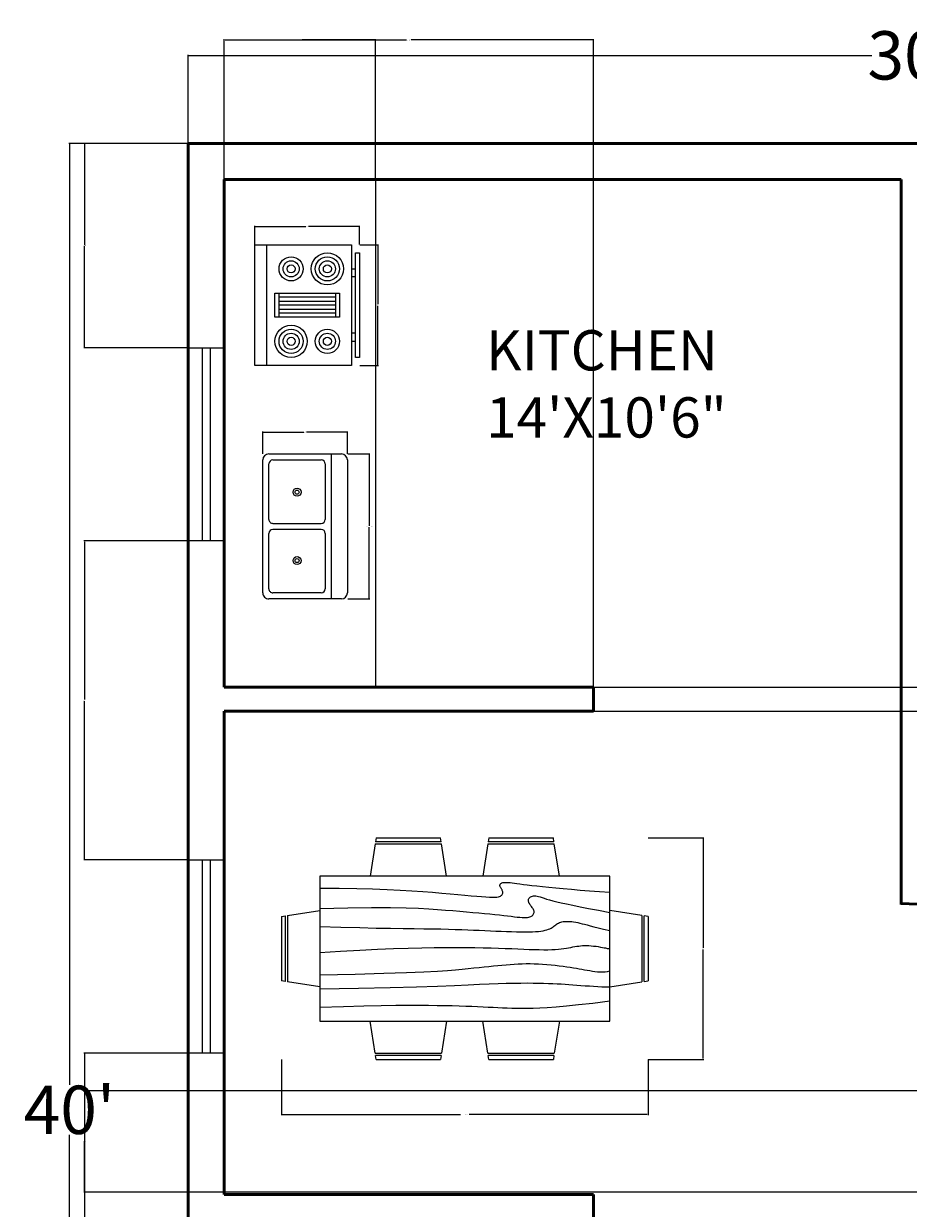
# Model space of a CAD drawing. Units: inches. Extents: x 471 to 898, y -3 to 533.
# Tile 2 of 3: x 471 to 691, y 239 to 533. Entities that reach past the tile are written whole.
import ezdxf

# ---------------------------------------------------------------- set-up
doc = ezdxf.new("R2010")
doc.units = ezdxf.units.IN
doc.header["$MEASUREMENT"] = 0
for name, color, linetype, lineweight in [('A-ANNO-DIMS', 2, 'Continuous', 18), ('A-AREA-IDEN', 7, 'Continuous', 25), ('A-EQPM', 8, 'Continuous', 18), ('A-FLOR-CASE', 8, 'Continuous', 25), ('A-FLOR-FIXT', 9, 'Continuous', 18), ('A-FURN', 8, 'Continuous', 18), ('A-GLAZ', 4, 'Continuous', 18), ('A-WALL', 7, 'Continuous', 50)]:
    doc.layers.add(name, color=color, linetype=linetype, lineweight=lineweight)
doc.styles.get("Standard").update_dxf_attribs({"font": 'arial.ttf'})
doc.dimstyles.get("Standard").update_dxf_attribs({"dimtxt": 0.18, "dimasz": 0.18, "dimexe": 0.18, "dimexo": 0.0625, "dimgap": 0.09, "dimtad": 0, "dimtih": 1, "dimtoh": 1, "dimdec": 1, "dimzin": 0, "dimdsep": 46, "dimlunit": 4, "dimtxsty": 'Standard', "dimcen": 0.09, "dimadec": 0, "dimazin": 0, "dimtfac": 1, "dimtdec": 1, "dimtofl": 0, "dimtmove": 0, "dimatfit": 3, "dimfxl": 1, "dimtolj": 1, "dimtzin": 0, "dimarcsym": 0})

# ---------------------------------------------------------------- blocks, each defined once
blk = doc.blocks.new('Range-Oven - 30 in top')
for p, q in [((0, -3), (30, -3)), ((12, -6), (18, -6)), ((13, -20), (13, -6)), ((14, -6), (14, -20)), ((15, -20), (15, -6)), ((16, -6), (16, -20)), ((17, -20), (17, -6)), ((18, -20), (12, -20)), ((6, -24), (6, -25)), ((8, -25), (8, -24)), ((22, -25), (22, -24)), ((24, -24), (24, -25))]:
    blk.add_line(p, q)
for points in [[(0, -24), (0, 0), (30, 0), (30, -24)], [(12, -21), (12, -5), (18, -5), (18, -21)], [(2, -26), (2, -25), (28, -25), (28, -26)]]:
    blk.add_lwpolyline(points, close=True)
for centre, radius in [((6, -9), 4), ((6, -9), 3), ((6, -9), 2), ((6, -9), 1), ((24, -9), 3), ((24, -9), 2), ((24, -9), 1), ((24, -18), 4), ((6, -18), 3), ((6, -18), 2), ((6, -18), 1), ((24, -18), 3), ((24, -18), 2), ((24, -18), 1)]:
    blk.add_circle(centre, radius)
blk = doc.blocks.new('Sink-double - 36 in top')
for p, q in [((-18, -4), (18, -4)), ((-0.75, -18.5), (-0.75, -6.5)), ((0.75, -6.5), (0.75, -18.5))]:
    blk.add_line(p, q)
for points in [[(-16.5, 0), (16.5, 0)], [(-18, -19.5), (-18, -1.5)], [(18, -1.5), (18, -19.5)], [(-15.5, -5.5), (-1.75, -5.5)], [(1.75, -5.5), (15.5, -5.5)], [(-16.5, -18.5), (-16.5, -6.5)], [(16.5, -6.5), (16.5, -18.5)], [(-1.75, -19.5), (-15.5, -19.5)], [(15.5, -19.5), (1.75, -19.5)], [(16.5, -21), (-16.5, -21)]]:
    blk.add_lwpolyline(points)
for centre, radius in [((-8.5, -12.5), 1), ((8.5, -12.5), 1), ((-8.5, -12.5), 0.5), ((8.5, -12.5), 0.5)]:
    blk.add_circle(centre, radius)
for centre, radius, start, end in [((-16.5, -1.5), 1.5, 90, 180), ((16.5, -1.5), 1.5, 0, 90), ((-15.5, -6.5), 1, 90, 180), ((-1.75, -6.5), 1, 0, 90), ((1.75, -6.5), 1, 90, 180), ((15.5, -6.5), 1, 0, 90), ((-16.5, -19.5), 1.5, 180, 270), ((-15.5, -18.5), 1, 180, 270), ((-1.75, -18.5), 1, 270, 0), ((1.75, -18.5), 1, 180, 270), ((15.5, -18.5), 1, 270, 0), ((16.5, -19.5), 1.5, 270, 0)]:
    blk.add_arc(centre, radius, start, end)
blk = doc.blocks.new('Dining Set - 36 x 72 in.')
for p, q in [((-22, 27.5), (-22.1562, 26.50042)), ((-5.8416, 26.5), (-22.1534, 26.5)), ((-22, 27.5), (-6, 27.5)), ((-5.8437, 26.49966), (-6, 27.5)), ((6, 27.5), (5.8438, 26.50042)), ((22.1584, 26.5), (5.8466, 26.5)), ((6, 27.5), (22, 27.5)), ((22.1563, 26.49966), (22, 27.5)), ((-22.2343, 26.00059), (-23.4847, 17.99762)), ((-22.2304, 26), (-5.7608, 26)), ((-4.5152, 17.99762), (-5.7655, 25.99926)), ((5.7657, 26.00059), (4.5153, 17.99762)), ((5.7696, 26), (22.2392, 26)), ((23.4848, 17.99762), (22.2345, 25.99926)), ((36, 18), (-36, 18)), ((-36, 18), (-36, -18)), ((36, -18), (36, 18)), ((-44.0006, 8.23428), (-35.9976, 9.48474)), ((44.0006, 8.23428), (35.9976, 9.48474)), ((-45.5, 8), (-44.5004, 8.15617)), ((-45.5, 8), (-45.5, -8)), ((-44.5, -8.15843), (-44.5, 8.15338)), ((-44, 8.23041), (-44, -8.23915)), ((44, 8.23041), (44, -8.23915)), ((44.5, -8.15843), (44.5, 8.15338)), ((45.5, 8), (44.5005, 8.15617)), ((45.5, 8), (45.5, -8)), ((-44.4997, -8.15631), (-45.5, -8)), ((-35.9976, -9.48476), (-43.9993, -8.2345)), ((35.9976, -9.48476), (43.9993, -8.2345)), ((44.4997, -8.15631), (45.5, -8)), ((-36, -18), (36, -18)), ((-22.2343, -26.0006), (-23.4847, -17.99762)), ((-4.5152, -17.99762), (-5.7655, -25.99928)), ((5.7657, -26.0006), (4.5153, -17.99762)), ((23.4848, -17.99762), (22.2345, -25.99928)), ((-22.2304, -26), (-5.7608, -26)), ((5.7696, -26), (22.2392, -26)), ((-22, -27.5), (-22.1562, -26.50044)), ((-5.8416, -26.5), (-22.1534, -26.5)), ((-22, -27.5), (-6, -27.5)), ((-5.8437, -26.49967), (-6, -27.5)), ((6, -27.5), (5.8438, -26.50044)), ((22.1584, -26.5), (5.8466, -26.5)), ((6, -27.5), (22, -27.5)), ((22.1563, -26.49967), (22, -27.5))]:
    blk.add_line(p, q)
for points in [[(-36, 15), (-31.1772, 14.97754), (-26.8079, 14.91406), (-22.8538, 14.81543), (-19.276, 14.6875), (-16.0362, 14.53613), (-13.0957, 14.36718), (-10.4159, 14.18652), (-7.9583, 14), (-5.6904, 13.81315), (-3.6035, 13.63021), (-1.6954, 13.45508), (0.0365, 13.29166), (1.5945, 13.14388), (2.9811, 13.01562), (4.1988, 12.9108), (5.25, 12.83333), (6.1393, 12.78613), (6.8802, 12.76823), (7.4883, 12.77767), (7.9792, 12.8125), (8.3685, 12.87077), (8.6719, 12.95052), (8.9049, 13.0498), (9.0833, 13.16666), (9.2205, 13.29899), (9.3216, 13.44401), (9.3895, 13.59879), (9.4271, 13.76041), (9.4373, 13.92594), (9.4232, 14.09245), (9.3875, 14.257), (9.3333, 14.41666), (9.2638, 14.56917), (9.1836, 14.71484), (9.0975, 14.85465), (9.0104, 14.98958), (8.9272, 15.1206), (8.8529, 15.2487), (8.7922, 15.37483), (8.75, 15.5), (8.7305, 15.62467), (8.7344, 15.74739), (8.7617, 15.86621), (8.8125, 15.97916), (8.8867, 16.08431), (8.9844, 16.17968), (9.1055, 16.26334), (9.25, 16.33333), (9.4189, 16.38802), (9.6172, 16.42708), (9.8506, 16.45052), (10.125, 16.45833), (10.4463, 16.45052), (10.8203, 16.42708), (11.2529, 16.38802), (11.75, 16.33333), (12.3184, 16.26318), (12.9694, 16.17838), (13.7151, 16.07991), (14.5677, 15.96875), (15.5395, 15.84586), (16.6426, 15.71224), (17.8893, 15.56884), (19.2917, 15.41666), (20.859, 15.25667), (22.5879, 15.08984), (24.4721, 14.91715), (26.5052, 14.73958), (28.6809, 14.5581), (30.9929, 14.3737), (33.4347, 14.18733), (36, 14)], [(-36, 10), (-28.9766, 10.14274), (-23.1725, 10.20442), (-18.4241, 10.19775), (-14.5677, 10.13541), (-11.4399, 10.03011), (-8.877, 9.89453), (-6.7154, 9.74137), (-4.7917, 9.58333), (-2.9698, 9.43082), (-1.2246, 9.28515), (0.4415, 9.14534), (2.026, 9.01041), (3.5266, 8.87939), (4.9408, 8.7513), (6.266, 8.62516), (7.5, 8.5), (8.6411, 8.37549), (9.6914, 8.2539), (10.6538, 8.13818), (11.5312, 8.03125), (12.3267, 7.93603), (13.043, 7.85547), (13.6831, 7.79248), (14.25, 7.75), (14.7471, 7.7303), (15.1797, 7.73307), (15.5537, 7.75732), (15.875, 7.80208), (16.1494, 7.86637), (16.3828, 7.94922), (16.5811, 8.04964), (16.75, 8.16666), (16.8944, 8.29915), (17.0143, 8.44531), (17.1089, 8.60319), (17.1771, 8.77083), (17.218, 8.94629), (17.2305, 9.1276), (17.2137, 9.31282), (17.1667, 9.5), (17.0895, 9.6875), (16.987, 9.875), (16.8649, 10.0625), (16.7292, 10.25), (16.5856, 10.4375), (16.4401, 10.625), (16.2985, 10.8125), (16.1667, 11), (16.05, 11.18733), (15.9518, 11.3737), (15.8752, 11.5581), (15.8229, 11.73958), (15.798, 11.91715), (15.8034, 12.08984), (15.842, 12.25667), (15.9167, 12.41666), (16.0295, 12.56836), (16.1784, 12.70833), (16.3605, 12.83268), (16.5729, 12.9375), (16.8127, 13.01888), (17.0768, 13.07291), (17.3625, 13.0957), (17.6667, 13.08333), (17.9894, 13.03312), (18.3418, 12.94726), (18.7382, 12.82918), (19.1927, 12.68229), (19.7195, 12.51001), (20.3327, 12.31575), (21.0465, 12.10294), (21.875, 11.875), (22.8357, 11.63354), (23.959, 11.37304), (25.2786, 11.08618), (26.8282, 10.76562), (28.6414, 10.40405), (30.752, 9.99414), (33.1936, 9.52856), (36, 9)], [(-36, 5.5), (-30.7157, 5.3348), (-26.069, 5.20963), (-21.9946, 5.11767), (-18.4271, 5.05208), (-15.3009, 5.00602), (-12.5508, 4.97265), (-10.1112, 4.94515), (-7.9167, 4.91666), (-5.909, 4.88167), (-4.0586, 4.83984), (-2.3429, 4.79215), (-0.7396, 4.73958), (0.7739, 4.6831), (2.22, 4.6237), (3.6213, 4.56233), (5, 4.5), (6.373, 4.43782), (7.7344, 4.3776), (9.0723, 4.32129), (10.375, 4.27083), (11.6309, 4.22819), (12.8281, 4.19531), (13.9551, 4.17415), (15, 4.16666), (15.954, 4.17448), (16.819, 4.19791), (17.6001, 4.23698), (18.3021, 4.29166), (18.9299, 4.36198), (19.4883, 4.44791), (19.9823, 4.54948), (20.4167, 4.66666), (20.7969, 4.79899), (21.1302, 4.94401), (21.4245, 5.09879), (21.6875, 5.26041), (21.9271, 5.42594), (22.1511, 5.59245), (22.3672, 5.757), (22.5834, 5.91666), (22.8065, 6.06868), (23.0404, 6.21093), (23.2879, 6.34147), (23.5521, 6.45833), (23.8358, 6.55957), (24.142, 6.64323), (24.4735, 6.70735), (24.8334, 6.75), (25.2235, 6.76969), (25.642, 6.76692), (26.0858, 6.74267), (26.5521, 6.69791), (27.0379, 6.63362), (27.5404, 6.55078), (28.0565, 6.45036), (28.5834, 6.33333), (29.1242, 6.19987), (29.7071, 6.04687), (30.3661, 5.87044), (31.1354, 5.66666), (32.0493, 5.43164), (33.142, 5.16146), (34.4475, 4.85221), (36, 4.5)], [(-36, -1), (-30.7915, -0.6591), (-26.0195, -0.38216), (-21.6519, -0.16284), (-17.6563, 0.00521), (-14.0005, 0.12833), (-10.6523, 0.21289), (-7.5796, 0.26522), (-4.75, 0.29166), (-2.134, 0.29793), (0.2878, 0.28711), (2.5317, 0.26163), (4.6146, 0.22396), (6.5529, 0.17651), (8.3633, 0.12174), (10.0623, 0.06209), (11.6667, 0), (13.1899, -0.06201), (14.6341, -0.1211), (15.9982, -0.17432), (17.2813, -0.21875), (18.4823, -0.25147), (19.6003, -0.26953), (20.6343, -0.27002), (21.5834, -0.25), (22.4481, -0.20768), (23.2357, -0.14584), (23.9549, -0.06836), (24.6146, 0.02083), (25.2235, 0.11784), (25.7904, 0.21875), (26.3241, 0.31966), (26.8334, 0.41666), (27.3265, 0.50618), (27.8099, 0.58593), (28.2894, 0.65397), (28.7709, 0.70833), (29.2601, 0.74707), (29.763, 0.76823), (30.2855, 0.76985), (30.8334, 0.75), (31.4088, 0.70784), (31.9994, 0.64713), (32.589, 0.57275), (33.1615, 0.48958), (33.7008, 0.4025), (34.1908, 0.3164), (34.6153, 0.23616), (34.9584, 0.16666), (35.2099, 0.11165), (35.3848, 0.07031), (35.504, 0.04069), (35.5886, 0.02083), (35.6594, 0.00879), (35.7377, 0.0026), (35.8442, 0.00032), (36, 0)], [(-36, -6.5), (-27.1843, -6.31267), (-20.084, -6.1263), (-14.469, -5.9419), (-10.1094, -5.76042), (-6.7752, -5.58285), (-4.2363, -5.41016), (-2.2629, -5.24333), (-0.625, -5.08334), (0.8708, -4.93099), (2.2715, -4.78646), (3.5872, -4.64974), (4.8281, -4.52084), (6.0046, -4.39974), (7.127, -4.28646), (8.2053, -4.18099), (9.25, -4.08334), (10.2705, -3.99382), (11.2734, -3.91407), (12.2647, -3.84603), (13.25, -3.79167), (14.2354, -3.75293), (15.2266, -3.73177), (16.2295, -3.73015), (17.25, -3.75), (18.2912, -3.79248), (19.3451, -3.85547), (20.4009, -3.93604), (21.4479, -4.03125), (22.4754, -4.13819), (23.4727, -4.25391), (24.4289, -4.37549), (25.3334, -4.5), (26.1785, -4.62492), (26.9694, -4.74935), (27.7145, -4.87281), (28.4219, -4.99479), (29.1, -5.11483), (29.7572, -5.23242), (30.4016, -5.34709), (31.0417, -5.45834), (31.6837, -5.56437), (32.3262, -5.65821), (32.9658, -5.73153), (33.599, -5.77604), (34.2224, -5.78345), (34.8327, -5.74545), (35.4264, -5.65373), (36, -5.5)], [(-36, -10), (-26.4022, -9.81299), (-18.4675, -9.62891), (-11.9839, -9.45069), (-6.7396, -9.28125), (-2.5226, -9.12354), (0.8789, -8.98047), (3.6769, -8.85498), (6.0833, -8.75), (8.2767, -8.66765), (10.3021, -8.60677), (12.1712, -8.56543), (13.8958, -8.54167), (15.4876, -8.53353), (16.9583, -8.53907), (18.3197, -8.55632), (19.5834, -8.58334), (20.7616, -8.61841), (21.8685, -8.66081), (22.9188, -8.71004), (23.9271, -8.76563), (24.9081, -8.82707), (25.8763, -8.89388), (26.8465, -8.96558), (27.8334, -9.04167), (28.8474, -9.12118), (29.8828, -9.20117), (30.93, -9.27824), (31.9792, -9.34896), (33.0205, -9.40991), (34.0443, -9.45768), (35.0407, -9.48885), (36, -9.5)], [(-36, -14.5), (-30.0881, -14.33513), (-25.0332, -14.21224), (-20.7312, -14.12647), (-17.0781, -14.07292), (-13.97, -14.04671), (-11.3027, -14.04297), (-8.9724, -14.05681), (-6.875, -14.08334), (-4.9224, -14.11833), (-3.0905, -14.16016), (-1.3709, -14.20785), (0.2448, -14.26042), (1.7647, -14.3169), (3.1973, -14.3763), (4.5507, -14.43767), (5.8333, -14.5), (7.0554, -14.5621), (8.235, -14.62175), (9.3922, -14.67652), (10.5469, -14.72396), (11.7192, -14.76164), (12.929, -14.78711), (14.1965, -14.79794), (15.5417, -14.79167), (16.9933, -14.76424), (18.6152, -14.70508), (20.4804, -14.60197), (22.6615, -14.44271), (25.2312, -14.21509), (28.2624, -13.9069), (31.8277, -13.50594), (36, -13)]]:
    blk.add_lwpolyline(points)
blk = doc.blocks.new('*D12')
at = {"layer": 'A-ANNO-DIMS', "color": 0, "lineweight": -2, "transparency": 16777216}
for p, q in [((512.23, 503.14), (512.23, 525.11)), ((512.41, 524.93), (681.96, 524.93)), ((872.05, 524.93), (702.5, 524.93)), ((872.23, 503.14), (872.23, 525.11))]:
    blk.add_line(p, q, dxfattribs=at)
at = {"layer": 'A-ANNO-DIMS', "color": 0, "transparency": 16777216}
for points in [[(512.41, 524.96), (512.41, 524.9), (512.23, 524.93)], [(872.05, 524.96), (872.05, 524.9), (872.23, 524.93)]]:
    blk.add_solid(points, dxfattribs=at)
at = {"layer": 'Defpoints', "color": 0, "transparency": 16777216}
for p in [(872.23, 524.93), (512.23, 503.07), (872.23, 503.07)]:
    blk.add_point(p, dxfattribs=at)
at = {"layer": 'A-ANNO-DIMS', "color": 0, "transparency": 16777216, "insert": (692.23, 524.93), "char_height": 12, "attachment_point": 5}
blk.add_mtext("\\A1;30'", dxfattribs=at)
blk = doc.blocks.new('*D13')
at = {"layer": 'A-ANNO-DIMS', "color": 0, "lineweight": -2, "transparency": 16777216}
for p, q in [((512.17, 503.07), (482.62, 503.07)), ((482.8, 502.89), (482.8, 269.29)), ((482.8, 23.25), (482.8, 256.86)), ((512.17, 23.07), (482.62, 23.07))]:
    blk.add_line(p, q, dxfattribs=at)
at = {"layer": 'A-ANNO-DIMS', "color": 0, "transparency": 16777216}
for points in [[(482.77, 502.89), (482.83, 502.89), (482.8, 503.07)], [(482.77, 23.25), (482.83, 23.25), (482.8, 23.07)]]:
    blk.add_solid(points, dxfattribs=at)
at = {"layer": 'Defpoints', "color": 0, "transparency": 16777216}
for p in [(512.23, 503.07), (482.8, 23.07), (512.23, 23.07)]:
    blk.add_point(p, dxfattribs=at)
at = {"layer": 'A-ANNO-DIMS', "color": 0, "transparency": 16777216, "insert": (482.8, 263.07), "char_height": 12, "attachment_point": 5}
blk.add_mtext("\\A1;40'", dxfattribs=at)
blk = doc.blocks.new('WIN-48X9')
for p, q in [((0, 48), (9, 48)), ((0, 0), (0, 48)), ((3.5, 48), (3.5, 0)), ((5.5, 48), (5.5, 0)), ((9, 48), (9, 0)), ((9, 0), (0, 0))]:
    blk.add_line(p, q)
blk = doc.blocks.new('*D23')
at = {"layer": 'A-ANNO-DIMS', "color": 0, "lineweight": -2, "transparency": 16777216}
for p, q in [((554.87, 477.92), (559.49, 477.92)), ((559.31, 477.74), (559.31, 463.11)), ((559.31, 448.1), (559.31, 462.74)), ((554.87, 447.92), (559.49, 447.92))]:
    blk.add_line(p, q, dxfattribs=at)
at = {"layer": 'A-ANNO-DIMS', "color": 0, "transparency": 16777216}
for points in [[(559.28, 477.74), (559.34, 477.74), (559.31, 477.92)], [(559.28, 448.1), (559.34, 448.1), (559.31, 447.92)]]:
    blk.add_solid(points, dxfattribs=at)
at = {"layer": 'Defpoints', "color": 0, "transparency": 16777216}
for p in [(554.81, 477.92), (559.31, 477.92), (554.81, 447.92)]:
    blk.add_point(p, dxfattribs=at)
at = {"layer": 'A-ANNO-DIMS', "color": 0, "transparency": 16777216, "insert": (559.31, 462.92), "char_height": 0.18, "attachment_point": 5}
blk.add_mtext('\\A1;RANGE 2\'-6"', dxfattribs=at)
blk = doc.blocks.new('*D24')
at = {"layer": 'A-ANNO-DIMS', "color": 0, "lineweight": -2, "transparency": 16777216}
for p, q in [((528.81, 477.99), (528.81, 482.6)), ((554.81, 477.99), (554.81, 482.6)), ((528.99, 482.42), (541.48, 482.42)), ((554.63, 482.42), (542.14, 482.42))]:
    blk.add_line(p, q, dxfattribs=at)
at = {"layer": 'A-ANNO-DIMS', "color": 0, "transparency": 16777216}
for points in [[(528.99, 482.45), (528.99, 482.39), (528.81, 482.42)], [(554.63, 482.45), (554.63, 482.39), (554.81, 482.42)]]:
    blk.add_solid(points, dxfattribs=at)
at = {"layer": 'Defpoints', "color": 0, "transparency": 16777216}
for p in [(528.81, 482.42), (528.81, 477.92), (554.81, 477.92)]:
    blk.add_point(p, dxfattribs=at)
at = {"layer": 'A-ANNO-DIMS', "color": 0, "transparency": 16777216, "insert": (541.81, 482.42), "char_height": 0.18, "attachment_point": 5}
blk.add_mtext('\\A1;2\'-2"', dxfattribs=at)
blk = doc.blocks.new('*D25')
at = {"layer": 'A-ANNO-DIMS', "color": 0, "lineweight": -2, "transparency": 16777216}
for p, q in [((551.85, 425.96), (557.37, 425.96)), ((557.19, 425.78), (557.19, 408.14)), ((557.19, 390.14), (557.19, 407.78)), ((551.85, 389.96), (557.37, 389.96))]:
    blk.add_line(p, q, dxfattribs=at)
at = {"layer": 'A-ANNO-DIMS', "color": 0, "transparency": 16777216}
for points in [[(557.16, 425.78), (557.22, 425.78), (557.19, 425.96)], [(557.16, 390.14), (557.22, 390.14), (557.19, 389.96)]]:
    blk.add_solid(points, dxfattribs=at)
at = {"layer": 'Defpoints', "color": 0, "transparency": 16777216}
for p in [(551.79, 425.96), (551.79, 389.96), (557.19, 389.96)]:
    blk.add_point(p, dxfattribs=at)
at = {"layer": 'A-ANNO-DIMS', "color": 0, "transparency": 16777216, "insert": (557.19, 407.96), "char_height": 0.18, "attachment_point": 5}
blk.add_mtext('\\A1;DOUBLE SINK 3\'-0"', dxfattribs=at)
blk = doc.blocks.new('*D26')
at = {"layer": 'A-ANNO-DIMS', "color": 0, "lineweight": -2, "transparency": 16777216}
for p, q in [((530.79, 426.02), (530.79, 431.54)), ((530.97, 431.36), (540.97, 431.36)), ((551.61, 431.36), (541.61, 431.36)), ((551.79, 426.02), (551.79, 431.54))]:
    blk.add_line(p, q, dxfattribs=at)
at = {"layer": 'A-ANNO-DIMS', "color": 0, "transparency": 16777216}
for points in [[(530.97, 431.39), (530.97, 431.33), (530.79, 431.36)], [(551.61, 431.39), (551.61, 431.33), (551.79, 431.36)]]:
    blk.add_solid(points, dxfattribs=at)
at = {"layer": 'Defpoints', "color": 0, "transparency": 16777216}
for p in [(551.79, 431.36), (530.79, 425.96), (551.79, 425.96)]:
    blk.add_point(p, dxfattribs=at)
at = {"layer": 'A-ANNO-DIMS', "color": 0, "transparency": 16777216, "insert": (541.29, 431.36), "char_height": 0.18, "attachment_point": 5}
blk.add_mtext('\\A1;1\'-9"', dxfattribs=at)
blk = doc.blocks.new('*D29')
at = {"layer": 'A-ANNO-DIMS', "color": 0, "lineweight": -2, "transparency": 16777216}
for p, q in [((535.4, 275.53), (535.4, 261.77)), ((626.4, 275.53), (626.4, 261.77)), ((535.58, 261.95), (579.82, 261.95)), ((626.22, 261.95), (581.98, 261.95))]:
    blk.add_line(p, q, dxfattribs=at)
at = {"layer": 'A-ANNO-DIMS', "color": 0, "transparency": 16777216}
for points in [[(535.58, 261.98), (535.58, 261.92), (535.4, 261.95)], [(626.22, 261.98), (626.22, 261.92), (626.4, 261.95)]]:
    blk.add_solid(points, dxfattribs=at)
at = {"layer": 'Defpoints', "color": 0, "transparency": 16777216}
for p in [(535.4, 275.6), (626.4, 275.6), (626.4, 261.95)]:
    blk.add_point(p, dxfattribs=at)
at = {"layer": 'A-ANNO-DIMS', "color": 0, "transparency": 16777216, "insert": (580.9, 261.95), "char_height": 0.18, "attachment_point": 5}
blk.add_mtext('\\A1;DINING SET 7\'-7"', dxfattribs=at)
blk = doc.blocks.new('*D30')
at = {"layer": 'A-ANNO-DIMS', "color": 0, "lineweight": -2, "transparency": 16777216}
for p, q in [((626.46, 330.6), (640.23, 330.6)), ((640.05, 330.42), (640.05, 303.28)), ((640.05, 275.78), (640.05, 302.92)), ((626.46, 275.6), (640.23, 275.6))]:
    blk.add_line(p, q, dxfattribs=at)
at = {"layer": 'A-ANNO-DIMS', "color": 0, "transparency": 16777216}
for points in [[(640.02, 330.42), (640.08, 330.42), (640.05, 330.6)], [(640.02, 275.78), (640.08, 275.78), (640.05, 275.6)]]:
    blk.add_solid(points, dxfattribs=at)
at = {"layer": 'Defpoints', "color": 0, "transparency": 16777216}
for p in [(626.4, 330.6), (640.05, 330.6), (626.4, 275.6)]:
    blk.add_point(p, dxfattribs=at)
at = {"layer": 'A-ANNO-DIMS', "color": 0, "transparency": 16777216, "insert": (640.05, 303.1), "char_height": 0.18, "attachment_point": 5}
blk.add_mtext('\\A1;4\'-7"', dxfattribs=at)
blk = doc.blocks.new('*D35')
at = {"layer": 'A-ANNO-DIMS', "color": 0, "lineweight": -2, "transparency": 16777216}
for p, q in [((512.17, 503.07), (486.35, 503.07)), ((486.53, 502.89), (486.53, 477.89)), ((486.53, 452.52), (486.53, 477.52)), ((512.17, 452.34), (486.35, 452.34))]:
    blk.add_line(p, q, dxfattribs=at)
at = {"layer": 'A-ANNO-DIMS', "color": 0, "transparency": 16777216}
for points in [[(486.5, 502.89), (486.56, 502.89), (486.53, 503.07)], [(486.5, 452.52), (486.56, 452.52), (486.53, 452.34)]]:
    blk.add_solid(points, dxfattribs=at)
at = {"layer": 'Defpoints', "color": 0, "transparency": 16777216}
for p in [(512.23, 503.07), (486.53, 452.34), (512.23, 452.34)]:
    blk.add_point(p, dxfattribs=at)
at = {"layer": 'A-ANNO-DIMS', "color": 0, "transparency": 16777216, "insert": (486.53, 477.71), "char_height": 0.18, "attachment_point": 5}
blk.add_mtext('\\A1;4\'-2 1/2"', dxfattribs=at)
blk = doc.blocks.new('*D36')
at = {"layer": 'A-ANNO-DIMS', "color": 0, "lineweight": -2, "transparency": 16777216}
for p, q in [((512.17, 404.34), (486.35, 404.34)), ((486.53, 404.16), (486.53, 364.94)), ((486.53, 325.36), (486.53, 364.58)), ((512.17, 325.18), (486.35, 325.18))]:
    blk.add_line(p, q, dxfattribs=at)
at = {"layer": 'A-ANNO-DIMS', "color": 0, "transparency": 16777216}
for points in [[(486.5, 404.16), (486.56, 404.16), (486.53, 404.34)], [(486.5, 325.36), (486.56, 325.36), (486.53, 325.18)]]:
    blk.add_solid(points, dxfattribs=at)
at = {"layer": 'Defpoints', "color": 0, "transparency": 16777216}
for p in [(512.23, 404.34), (486.53, 325.18), (512.23, 325.18)]:
    blk.add_point(p, dxfattribs=at)
at = {"layer": 'A-ANNO-DIMS', "color": 0, "transparency": 16777216, "insert": (486.53, 364.76), "char_height": 0.18, "attachment_point": 5}
blk.add_mtext('\\A1;6\'-7"', dxfattribs=at)
blk = doc.blocks.new('*D37')
at = {"layer": 'A-ANNO-DIMS', "color": 0, "lineweight": -2, "transparency": 16777216}
for p, q in [((512.17, 277.18), (486.35, 277.18)), ((486.53, 277), (486.53, 214.23)), ((486.53, 151.09), (486.53, 213.86)), ((512.17, 150.91), (486.35, 150.91))]:
    blk.add_line(p, q, dxfattribs=at)
at = {"layer": 'A-ANNO-DIMS', "color": 0, "transparency": 16777216}
for points in [[(486.5, 277), (486.56, 277), (486.53, 277.18)], [(486.5, 151.09), (486.56, 151.09), (486.53, 150.91)]]:
    blk.add_solid(points, dxfattribs=at)
at = {"layer": 'Defpoints', "color": 0, "transparency": 16777216}
for p in [(512.23, 277.18), (486.53, 150.91), (512.23, 150.91)]:
    blk.add_point(p, dxfattribs=at)
at = {"layer": 'A-ANNO-DIMS', "color": 0, "transparency": 16777216, "insert": (486.53, 214.04), "char_height": 0.18, "attachment_point": 5}
blk.add_mtext('\\A1;10\'-6 1/2"', dxfattribs=at)
blk = doc.blocks.new('*D44')
at = {"layer": 'A-ANNO-DIMS', "color": 0, "lineweight": -2, "transparency": 16777216}
for p, q in [((521.23, 368.14), (521.23, 528.95)), ((521.41, 528.77), (566.49, 528.77)), ((612.65, 528.77), (567.57, 528.77)), ((612.83, 368.14), (612.83, 528.95))]:
    blk.add_line(p, q, dxfattribs=at)
at = {"layer": 'A-ANNO-DIMS', "color": 0, "transparency": 16777216}
for points in [[(521.41, 528.8), (521.41, 528.74), (521.23, 528.77)], [(612.65, 528.8), (612.65, 528.74), (612.83, 528.77)]]:
    blk.add_solid(points, dxfattribs=at)
at = {"layer": 'Defpoints', "color": 0, "transparency": 16777216}
for p in [(612.83, 528.77), (521.23, 368.07), (612.83, 368.07)]:
    blk.add_point(p, dxfattribs=at)
at = {"layer": 'A-ANNO-DIMS', "color": 0, "transparency": 16777216, "insert": (567.03, 528.77), "char_height": 0.18, "attachment_point": 5}
blk.add_mtext('\\A1;7\'-7 1/2"', dxfattribs=at)
blk = doc.blocks.new('*D45')
at = {"layer": 'A-ANNO-DIMS', "color": 0, "lineweight": -2, "transparency": 16777216}
for p, q in [((612.9, 368.07), (898.15, 368.07)), ((897.97, 367.89), (897.97, 365.26)), ((897.97, 362.25), (897.97, 364.89)), ((612.9, 362.07), (898.15, 362.07))]:
    blk.add_line(p, q, dxfattribs=at)
at = {"layer": 'A-ANNO-DIMS', "color": 0, "transparency": 16777216}
for points in [[(897.94, 367.89), (898, 367.89), (897.97, 368.07)], [(897.94, 362.25), (898, 362.25), (897.97, 362.07)]]:
    blk.add_solid(points, dxfattribs=at)
at = {"layer": 'Defpoints', "color": 0, "transparency": 16777216}
for p in [(612.83, 368.07), (897.97, 368.07), (612.83, 362.07)]:
    blk.add_point(p, dxfattribs=at)
at = {"layer": 'A-ANNO-DIMS', "color": 0, "transparency": 16777216, "insert": (897.97, 365.07), "char_height": 0.18, "attachment_point": 5}
blk.add_mtext('\\A1;0\'-6"', dxfattribs=at)
blk = doc.blocks.new('*D47')
at = {"layer": 'A-ANNO-DIMS', "color": 0, "lineweight": -2, "transparency": 16777216}
for p, q in [((521.23, 494.14), (521.23, 528.95)), ((521.41, 528.77), (539.45, 528.77)), ((558.56, 528.77), (540.53, 528.77)), ((558.74, 494.14), (558.74, 528.95))]:
    blk.add_line(p, q, dxfattribs=at)
at = {"layer": 'A-ANNO-DIMS', "color": 0, "transparency": 16777216}
for points in [[(521.41, 528.8), (521.41, 528.74), (521.23, 528.77)], [(558.56, 528.8), (558.56, 528.74), (558.74, 528.77)]]:
    blk.add_solid(points, dxfattribs=at)
at = {"layer": 'Defpoints', "color": 0, "transparency": 16777216}
for p in [(558.74, 528.77), (521.23, 494.07), (558.74, 494.07)]:
    blk.add_point(p, dxfattribs=at)
at = {"layer": 'A-ANNO-DIMS', "color": 0, "transparency": 16777216, "insert": (539.99, 528.77), "char_height": 0.18, "attachment_point": 5}
blk.add_mtext('\\A1;3\'-1 1/2"', dxfattribs=at)
blk = doc.blocks.new('*D50')
at = {"layer": 'A-ANNO-DIMS', "color": 0, "lineweight": -2, "transparency": 16777216}
for p, q in [((785.17, 267.78), (486.35, 267.78)), ((486.53, 267.6), (486.53, 255.39)), ((486.53, 242.81), (486.53, 255.03)), ((791.03, 242.63), (486.35, 242.63))]:
    blk.add_line(p, q, dxfattribs=at)
at = {"layer": 'A-ANNO-DIMS', "color": 0, "transparency": 16777216}
for points in [[(486.5, 267.6), (486.56, 267.6), (486.53, 267.78)], [(486.5, 242.81), (486.56, 242.81), (486.53, 242.63)]]:
    blk.add_solid(points, dxfattribs=at)
at = {"layer": 'Defpoints', "color": 0, "transparency": 16777216}
for p in [(486.53, 267.78), (785.23, 267.78), (791.1, 242.63)]:
    blk.add_point(p, dxfattribs=at)
at = {"layer": 'A-ANNO-DIMS', "color": 0, "transparency": 16777216, "insert": (486.53, 255.21), "char_height": 0.18, "attachment_point": 5}
blk.add_mtext('\\A1;2\'-1"', dxfattribs=at)

msp = doc.modelspace()

# ---------------------------------------------------------------- linework, layer by layer
at = {"layer": 'A-FLOR-CASE'}
msp.add_line((558.74, 494.07), (558.74, 368.07), dxfattribs=at)
at = {"layer": 'A-WALL'}
for p, q in [((512.23, 23.07), (512.23, 503.07)), ((512.23, 503.07), (872.23, 503.07)), ((521.23, 494.07), (689.23, 494.07)), ((521.23, 494.07), (689.23, 494.07)), ((521.23, 368.07), (521.23, 494.07)), ((689.23, 494.07), (689.23, 320.07)), ((612.83, 368.07), (521.23, 368.07)), ((612.83, 368.07), (612.83, 362.07)), ((612.83, 362.07), (521.23, 362.07)), ((521.23, 242.07), (521.23, 362.07)), ((689.23, 362.07), (689.23, 314.07)), ((695.23, 314.07), (689.23, 314.28)), ((612.83, 242.07), (521.23, 242.07)), ((612.83, 242.07), (612.83, 236.07))]:
    msp.add_line(p, q, dxfattribs=at)

# ---------------------------------------------------------------- block references
at = {"layer": 'A-EQPM', "rotation": 90}
msp.add_blockref('Range-Oven - 30 in top', (528.81, 447.92), dxfattribs=at)
at = {"layer": 'A-FLOR-FIXT', "rotation": 270}
msp.add_blockref('Sink-double - 36 in top', (551.79, 407.96), dxfattribs=at)
at = {"layer": 'A-FURN'}
msp.add_blockref('Dining Set - 36 x 72 in.', (580.9, 303.1), dxfattribs=at)
at = {"layer": 'A-GLAZ'}
for p in [(512.23, 404.34), (512.23, 277.18)]:
    msp.add_blockref('WIN-48X9', p, dxfattribs=at)

# ---------------------------------------------------------------- texts
at = {"layer": 'A-AREA-IDEN', "insert": (586.21, 456.69), "char_height": 10, "attachment_point": 1}
msp.add_mtext_dynamic_manual_height_columns('KITCHEN\\P14\'X10\'6"', width=80.8054, gutter_width=1, heights=[0], dxfattribs=at)

# ---------------------------------------------------------------- dimensions: what is measured, and where the dimension line sits
at = {"layer": 'A-ANNO-DIMS'}
for base, p1, p2, override, picture, middle in [((872.23, 524.93), (512.23, 503.07), (872.23, 503.07), {"dimtxt": 12, "dimclrd": 0, "dimclre": 0, "dimclrt": 0}, '*D12', (692.23, 524.93)), ((612.83, 528.77), (521.23, 368.07), (612.83, 368.07), {"dimdec": 1, "dimlfac": 1, "dimrnd": 0, "dimzin": 1, "dimdsep": 46, "dimlunit": 4, "dimfrac": 2}, '*D44', (567.03, 528.77)), ((558.74, 528.77), (521.23, 494.07), (558.74, 494.07), {"dimdec": 1, "dimlfac": 1, "dimrnd": 0, "dimzin": 1, "dimdsep": 46, "dimlunit": 4, "dimfrac": 2}, '*D47', (539.99, 528.77)), ((551.79, 431.36), (530.79, 425.96), (551.79, 425.96), {"dimdec": 1, "dimlfac": 1, "dimrnd": 0, "dimzin": 1, "dimdsep": 46, "dimlunit": 4, "dimfrac": 2}, '*D26', (541.29, 431.36))]:
    dim = msp.add_linear_dim(base=base, p1=p1, p2=p2, dimstyle='Standard', override=override, dxfattribs=at)
    dim.commit()
    dim.dimension.update_dxf_attribs({"geometry": picture, "text_midpoint": middle})
for base, p1, p2, angle, override, picture, middle in [((482.8, 23.07), (512.23, 503.07), (512.23, 23.07), 90, {"dimtxt": 12, "dimclrd": 0, "dimclre": 0, "dimclrt": 0}, '*D13', (482.8, 263.07)), ((486.53, 452.34), (512.23, 503.07), (512.23, 452.34), 90, {"dimdec": 1, "dimlfac": 1, "dimrnd": 0, "dimzin": 1, "dimdsep": 46, "dimlunit": 4, "dimfrac": 2}, '*D35', (486.53, 477.71)), ((528.81, 482.42), (554.81, 477.92), (528.81, 477.92), 180, {"dimdec": 1, "dimlfac": 1, "dimrnd": 0, "dimzin": 1, "dimdsep": 46, "dimlunit": 4, "dimfrac": 2}, '*D24', (541.81, 482.42)), ((486.53, 325.18), (512.23, 404.34), (512.23, 325.18), 90, {"dimdec": 1, "dimlfac": 1, "dimrnd": 0, "dimzin": 1, "dimdsep": 46, "dimlunit": 4, "dimfrac": 2}, '*D36', (486.53, 364.76)), ((897.97, 368.07), (612.83, 362.07), (612.83, 368.07), 90, {"dimdec": 1, "dimlfac": 1, "dimrnd": 0, "dimzin": 1, "dimdsep": 46, "dimlunit": 4, "dimfrac": 2}, '*D45', (897.97, 365.07)), ((640.05, 330.6), (626.4, 275.6), (626.4, 330.6), 90, {"dimdec": 1, "dimlfac": 1, "dimrnd": 0, "dimzin": 1, "dimdsep": 46, "dimlunit": 4, "dimfrac": 2}, '*D30', (640.05, 303.1)), ((486.53, 150.91), (512.23, 277.18), (512.23, 150.91), 90, {"dimdec": 1, "dimlfac": 1, "dimrnd": 0, "dimzin": 1, "dimdsep": 46, "dimlunit": 4, "dimfrac": 2}, '*D37', (486.53, 214.04)), ((486.532, 267.7812), (791.0957, 242.6327), (785.232, 267.7812), 90, {"dimdec": 1, "dimlfac": 1, "dimrnd": 0, "dimzin": 1, "dimdsep": 46, "dimlunit": 4, "dimfrac": 2}, '*D50', (486.532, 255.207))]:
    dim = msp.add_linear_dim(base=base, p1=p1, p2=p2, angle=angle, dimstyle='Standard', override=override, dxfattribs=at)
    dim.commit()
    dim.dimension.update_dxf_attribs({"geometry": picture, "text_midpoint": middle})
for base, p1, p2, angle, text, picture, middle in [((559.31, 477.92), (554.81, 447.92), (554.81, 477.92), 90, 'RANGE <>', '*D23', (559.31, 462.92)), ((557.19, 389.96), (551.79, 425.96), (551.79, 389.96), 270, 'DOUBLE SINK <>', '*D25', (557.19, 407.96))]:
    dim = msp.add_linear_dim(base=base, p1=p1, p2=p2, angle=angle, text=text, dimstyle='Standard', override={"dimdec": 1, "dimlfac": 1, "dimrnd": 0, "dimzin": 1, "dimdsep": 46, "dimlunit": 4, "dimfrac": 2}, dxfattribs=at)
    dim.commit()
    dim.dimension.update_dxf_attribs({"geometry": picture, "text_midpoint": middle})
dim = msp.add_linear_dim(base=(626.4, 261.95), p1=(535.4, 275.6), p2=(626.4, 275.6), text='DINING SET <>', dimstyle='Standard', override={"dimdec": 1, "dimlfac": 1, "dimrnd": 0, "dimzin": 1, "dimdsep": 46, "dimlunit": 4, "dimfrac": 2}, dxfattribs=at)
dim.commit()
dim.dimension.update_dxf_attribs({"geometry": '*D29', "text_midpoint": (580.9, 261.95)})

doc.saveas('drawing.dxf')
